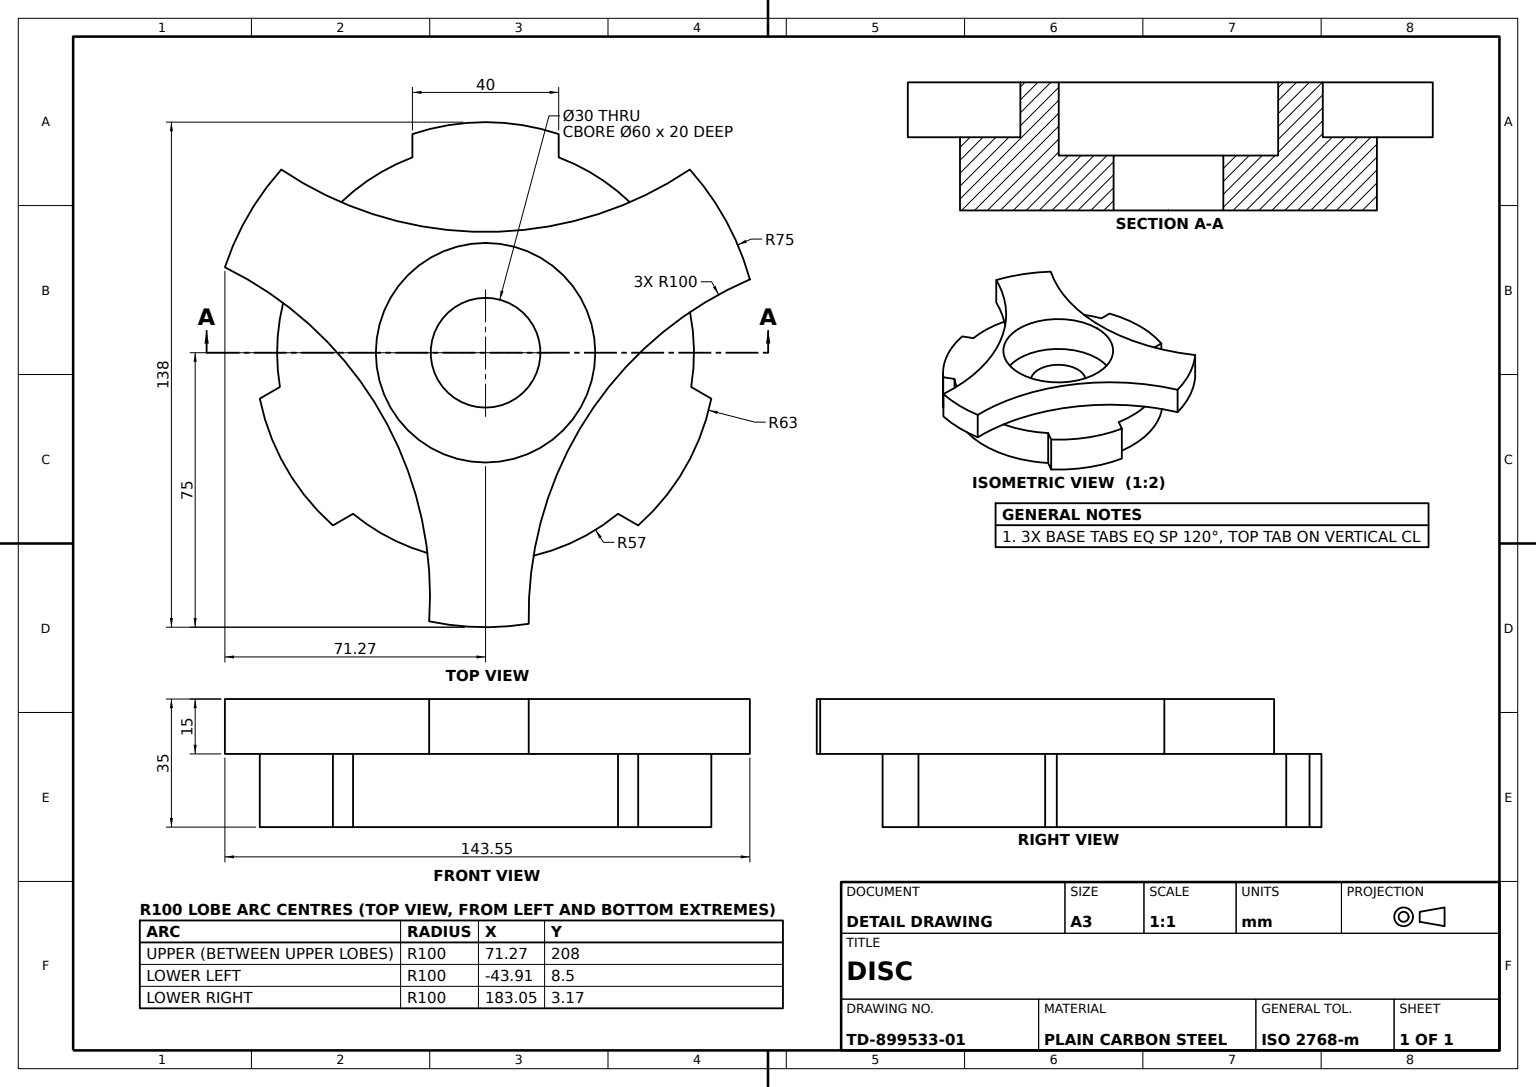
SolidWorks part; units mm, degrees
material "Plain Carbon Steel"
ref_plane "Front Plane" through (0, 0, 0) normal (0, 0, 1) x (1, 0, 0)
ref_plane "Top Plane" through (0, 0, 0) normal (0, 1, 0) x (1, 0, 0)
ref_plane "Right Plane" through (0, 0, 0) normal (1, 0, 0) x (0, 0, -1)
sketch "Base Disc Profile" plane through (0, 0, 0) normal (0, 1, 0) x (1, 0, 0)
  line L0 (0, 63) -> (0, -63) construction
  line L1 (-63, 0) -> (65.6711, 0) construction
  line L3 (-20, 53.376) -> (-20, 59.7411)
  line L4 (20, 53.376) -> (20, 59.7411)
  line L5 (0, 0) -> (-54.5596, -31.5) construction
  line L6 (0, 0) -> (54.5596, -31.5) construction
  line L7 (56.225, -9.3675) -> (61.7373, -12.55)
  line L8 (-36.225, -44.0085) -> (-41.7373, -47.1911)
  line L10 (36.225, -44.0085) -> (41.7373, -47.1911)
  line L13 (-56.225, -9.3675) -> (-61.7373, -12.55)
  arc A6 (-61.7373, -12.55) -> (-41.7373, -47.1911) centre (0, 0) ccw
  arc A7 (-36.225, -44.0085) -> (36.225, -44.0085) centre (0, 0) ccw
  arc A12 (-20, 53.376) -> (-56.225, -9.3675) centre (0, 0) ccw
  arc A16 (56.225, -9.3675) -> (20, 53.376) centre (0, 0) ccw
  arc A17 (41.7373, -47.1911) -> (61.7373, -12.55) centre (0, 0) ccw
  arc A18 (20, 59.7411) -> (-20, 59.7411) centre (0, 0) ccw
  dimension "D1" = 63
  dimension "D2" = 57
  dimension "D3" = 20
  dimension "D4" = 56.225
  dimension "D5" = 76.225
extrude "Base Disc 20mm" add sketch "Base Disc Profile" along normal blind 20
sketch "Three-Lobe Profile" plane through (0, 20, 0) normal (0, 1, 0) x (1, 0, 0)
  line L0 (0, 63) -> (0, 133) construction
  line L1 (-54.5596, -31.5) -> (-115.1814, -66.5) construction
  line L2 (54.5596, -31.5) -> (111.7767, -71.8262) construction
  arc A0 (-55.8546, 50.0526) -> (-71.2741, 23.3452) centre (0, 0) ccw
  arc A1 (-49.8125, 46.2895) -> (-64.9941, 19.9941) centre (0, 0) ccw
  arc A2 (20, 59.7411) -> (-20, 59.7411) centre (0, 0) ccw construction
  arc A3 (-55.8546, 50.0526) -> (55.8546, 50.0526) centre (0, 133) ccw
  arc A4 (-61.7373, -12.55) -> (-41.7373, -47.1911) centre (0, 0) ccw construction
  arc A5 (41.7373, -47.1911) -> (61.7373, -12.55) centre (0, 0) ccw construction
  arc A6 (-15.4196, -73.3978) -> (-71.2741, 23.3452) centre (-115.1814, -66.5) ccw
  arc A7 (72.273, 20.0403) -> (11.8018, -74.0656) centre (111.7767, -71.8262) ccw
  arc A8 (65.841, 16.999) -> (49.8125, 46.2895) centre (0, 0) ccw
  arc A9 (72.273, 20.0403) -> (55.8546, 50.0526) centre (0, 0) ccw
  arc A10 (-15.4196, -73.3978) -> (11.8018, -74.0656) centre (0, 0) ccw
  arc A11 (-15.1816, -66.2836) -> (11.8956, -66.9514) centre (0, 0) ccw
  arc M1 (-20, 53.376) -> (-56.225, -9.3675) centre (0, 0) ccw
  arc M5 (-36.225, -44.0085) -> (36.225, -44.0085) centre (0, 0) ccw
  arc M9 (56.225, -9.3675) -> (20, 53.376) centre (0, 0) ccw
  dimension "D1" = 75
  dimension "D2" = 68
  dimension "D3" = 100
  dimension "D4" = 8.0752
  dimension "D5" = 24.1037
extrude "Three-Lobe Boss 15mm" add sketch "Three-Lobe Profile" along normal blind 15 contours A7 A3 A6 M9 M1 M5 | A6 A3 A1 M1 | A6 A1 A3 A0 | A6 A11 A7 M5 | A11 A6 A10 A7 | A7 A8 A3 M9 | A7 A9 A3 A8
sketch "Counterbore Profile" plane through (0, 35, 0) normal (0, 1, 0) x (1, 0, 0)
  circle A0 centre (0, 0) radius 30
  dimension "D1" = 60
extrude "Counterbore 20mm Deep" cut sketch "Counterbore Profile" against normal blind 20
sketch "Through Bore Profile" plane through (0, 15, 0) normal (0, 1, 0) x (1, 0, 0)
  circle A0 centre (0, 0) radius 15
  dimension "D1" = 30
extrude "Through Bore" cut sketch "Through Bore Profile" against normal through all
